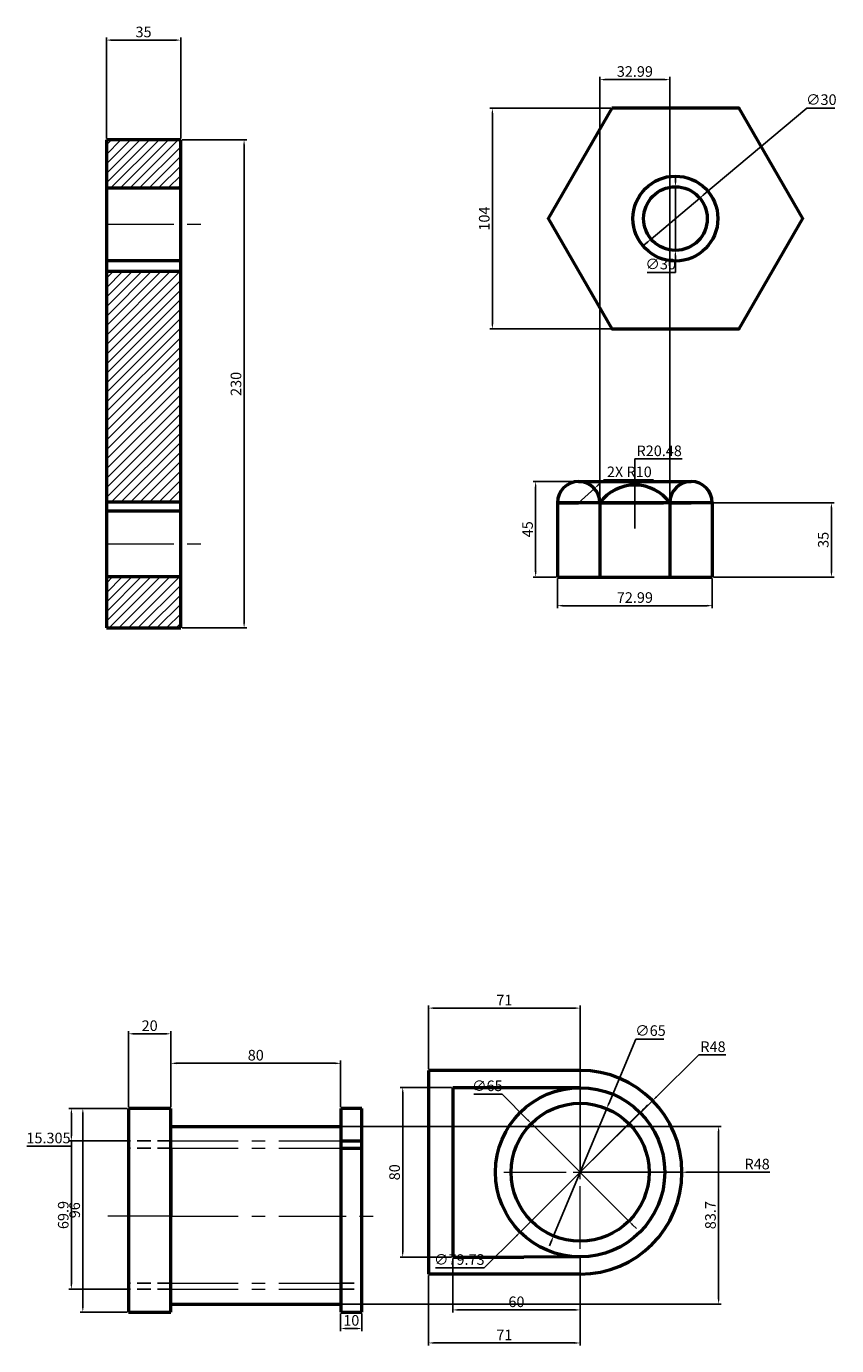
# Model space of a CAD drawing. Units: millimetres. Extents: x 1084 to 2343, y 1141 to 1965.
# Tile 4 of 4: x 1961 to 2343, y 1321 to 1942. Entities that reach past the tile are written whole.
import ezdxf

# ---------------------------------------------------------------- set-up
doc = ezdxf.new("R2010")
doc.units = ezdxf.units.MM
doc.linetypes.add('CENTER', pattern=[50.8, 31.75, -6.35, 6.35, -6.35])
doc.linetypes.add('HIDDEN', pattern=[9.525, 6.35, -3.175])
for name, color, linetype, lineweight in [('M-CNTR', 1, 'CENTER', 18), ('M-DIMS', 2, 'Continuous', 25), ('M-HATC', 8, 'Continuous', 18), ('M-HIDN', 8, 'HIDDEN', 25), ('M-OUTL', 7, 'Continuous', 50)]:
    doc.layers.add(name, color=color, linetype=linetype, lineweight=lineweight)
doc.styles.get("Standard").update_dxf_attribs({"font": 'arial.ttf'})
doc.dimstyles.new('ISO-25', dxfattribs={"dimtxt": 5, "dimasz": 2.5, "dimexe": 1.25, "dimexo": 0.625, "dimtad": 1, "dimtoh": 1, "dimdec": 0, "dimtxsty": 'Standard', "dimcen": 2.5, "dimadec": 0, "dimazin": 0, "dimtfac": 1, "dimtdec": 0, "dimtmove": 0, "dimatfit": 3, "dimfxl": 1, "dimarcsym": 0})

# ---------------------------------------------------------------- blocks, each defined once
blk = doc.blocks.new('*D21')
at = {"layer": 'Defpoints', "color": 0, "transparency": 16777216}
for p in [(2033.5, 1935.59), (1998.5, 1888.61), (2033.5, 1888.61)]:
    blk.add_point(p, dxfattribs=at)
at = {"layer": 'M-DIMS', "color": 0, "lineweight": -2, "transparency": 16777216}
for p, q in [((1998.5, 1889.24), (1998.5, 1936.84)), ((2001, 1935.59), (2031, 1935.59)), ((2033.5, 1889.24), (2033.5, 1936.84))]:
    blk.add_line(p, q, dxfattribs=at)
at = {"layer": 'M-DIMS', "color": 0, "transparency": 16777216}
for points in [[(2001, 1936), (2001, 1935.17), (1998.5, 1935.59)], [(2031, 1936), (2031, 1935.17), (2033.5, 1935.59)]]:
    blk.add_solid(points, dxfattribs=at)
at = {"layer": 'M-DIMS', "color": 0, "transparency": 16777216, "insert": (2016, 1938.77), "char_height": 5, "attachment_point": 5}
blk.add_mtext('35', dxfattribs=at)
blk = doc.blocks.new('*D22')
at = {"layer": 'Defpoints', "color": 0, "transparency": 16777216}
for p in [(2236.62, 1903.46), (2180.37, 1799.54), (2236.62, 1799.54)]:
    blk.add_point(p, dxfattribs=at)
at = {"layer": 'M-DIMS', "color": 0, "lineweight": -2, "transparency": 16777216}
for p, q in [((2236, 1903.46), (2179.12, 1903.46)), ((2180.37, 1900.96), (2180.37, 1802.04)), ((2236, 1799.54), (2179.12, 1799.54))]:
    blk.add_line(p, q, dxfattribs=at)
at = {"layer": 'M-DIMS', "color": 0, "transparency": 16777216}
for points in [[(2179.95, 1900.96), (2180.79, 1900.96), (2180.37, 1903.46)], [(2179.95, 1802.04), (2180.79, 1802.04), (2180.37, 1799.54)]]:
    blk.add_solid(points, dxfattribs=at)
at = {"layer": 'M-DIMS', "color": 0, "transparency": 16777216, "insert": (2177.19, 1851.5), "char_height": 5, "attachment_point": 5, "rotation": 90}
blk.add_mtext('104', dxfattribs=at)
blk = doc.blocks.new('*D23')
at = {"layer": 'Defpoints', "color": 0, "transparency": 16777216}
for p in [(2278.1, 1861.16), (2255.15, 1841.84)]:
    blk.add_point(p, dxfattribs=at)
at = {"layer": 'M-DIMS', "color": 0, "lineweight": -2, "transparency": 16777216}
for p, q in [((2328.46, 1903.58), (2280.01, 1862.77)), ((2341.67, 1903.58), (2328.46, 1903.58)), ((2255.15, 1841.84), (2278.1, 1861.16)), ((2253.24, 1840.23), (2251.33, 1838.62))]:
    blk.add_line(p, q, dxfattribs=at)
at = {"layer": 'M-DIMS', "color": 0, "transparency": 16777216}
for points in [[(2279.74, 1863.09), (2280.28, 1862.46), (2278.1, 1861.16)], [(2252.97, 1840.55), (2253.51, 1839.91), (2255.15, 1841.84)]]:
    blk.add_solid(points, dxfattribs=at)
at = {"layer": 'M-DIMS', "color": 0, "transparency": 16777216, "insert": (2335.37, 1906.89), "char_height": 5, "attachment_point": 5}
blk.add_mtext('∅30', dxfattribs=at)
blk = doc.blocks.new('*D24')
at = {"layer": 'Defpoints', "color": 0, "transparency": 16777216}
for p in [(2221.01, 1727.62), (2200.76, 1682.62), (2211.01, 1682.62)]:
    blk.add_point(p, dxfattribs=at)
at = {"layer": 'M-DIMS', "color": 0, "lineweight": -2, "transparency": 16777216}
for p, q in [((2220.39, 1727.62), (2199.51, 1727.62)), ((2200.76, 1725.12), (2200.76, 1685.12)), ((2210.39, 1682.62), (2199.51, 1682.62))]:
    blk.add_line(p, q, dxfattribs=at)
at = {"layer": 'M-DIMS', "color": 0, "transparency": 16777216}
for points in [[(2200.35, 1725.12), (2201.18, 1725.12), (2200.76, 1727.62)], [(2200.35, 1685.12), (2201.18, 1685.12), (2200.76, 1682.62)]]:
    blk.add_solid(points, dxfattribs=at)
at = {"layer": 'M-DIMS', "color": 0, "transparency": 16777216, "insert": (2197.59, 1705.12), "char_height": 5, "attachment_point": 5, "rotation": 90}
blk.add_mtext('45', dxfattribs=at)
blk = doc.blocks.new('*D38')
at = {"layer": 'Defpoints', "color": 0, "transparency": 16777216}
for p in [(2008.88, 1432.29), (1987.38, 1336.29), (2008.88, 1336.29)]:
    blk.add_point(p, dxfattribs=at)
at = {"layer": 'M-DIMS', "color": 0, "lineweight": -2, "transparency": 16777216}
for p, q in [((2008.26, 1432.29), (1986.13, 1432.29)), ((1987.38, 1429.79), (1987.38, 1338.79)), ((2008.26, 1336.29), (1986.13, 1336.29))]:
    blk.add_line(p, q, dxfattribs=at)
at = {"layer": 'M-DIMS', "color": 0, "transparency": 16777216}
for points in [[(1986.97, 1429.79), (1987.8, 1429.79), (1987.38, 1432.29)], [(1986.97, 1338.79), (1987.8, 1338.79), (1987.38, 1336.29)]]:
    blk.add_solid(points, dxfattribs=at)
at = {"layer": 'M-DIMS', "color": 0, "transparency": 16777216, "insert": (1984.2, 1384.29), "char_height": 5, "attachment_point": 5, "rotation": 90}
blk.add_mtext('96', dxfattribs=at)
blk = doc.blocks.new('*D39')
at = {"layer": 'Defpoints', "color": 0, "transparency": 16777216}
for p in [(2108.88, 1453.51), (2028.88, 1432.29), (2108.88, 1432.29)]:
    blk.add_point(p, dxfattribs=at)
at = {"layer": 'M-DIMS', "color": 0, "lineweight": -2, "transparency": 16777216}
for p, q in [((2028.88, 1432.92), (2028.88, 1454.76)), ((2108.88, 1432.92), (2108.88, 1454.76)), ((2031.38, 1453.51), (2106.38, 1453.51))]:
    blk.add_line(p, q, dxfattribs=at)
at = {"layer": 'M-DIMS', "color": 0, "transparency": 16777216}
for points in [[(2031.38, 1453.93), (2031.38, 1453.09), (2028.88, 1453.51)], [(2106.38, 1453.93), (2106.38, 1453.09), (2108.88, 1453.51)]]:
    blk.add_solid(points, dxfattribs=at)
at = {"layer": 'M-DIMS', "color": 0, "transparency": 16777216, "insert": (2068.88, 1456.69), "char_height": 5, "attachment_point": 5}
blk.add_mtext('80', dxfattribs=at)
blk = doc.blocks.new('*D40')
at = {"layer": 'Defpoints', "color": 0, "transparency": 16777216}
for p in [(2108.88, 1336.29), (2118.88, 1336.29), (2118.88, 1328.57)]:
    blk.add_point(p, dxfattribs=at)
at = {"layer": 'M-DIMS', "color": 0, "lineweight": -2, "transparency": 16777216}
for p, q in [((2108.88, 1335.67), (2108.88, 1327.32)), ((2118.88, 1335.67), (2118.88, 1327.32)), ((2111.38, 1328.57), (2116.38, 1328.57))]:
    blk.add_line(p, q, dxfattribs=at)
at = {"layer": 'M-DIMS', "color": 0, "transparency": 16777216}
for points in [[(2111.38, 1328.98), (2111.38, 1328.15), (2108.88, 1328.57)], [(2116.38, 1328.98), (2116.38, 1328.15), (2118.88, 1328.57)]]:
    blk.add_solid(points, dxfattribs=at)
at = {"layer": 'M-DIMS', "color": 0, "transparency": 16777216, "insert": (2113.88, 1331.75), "char_height": 5, "attachment_point": 5}
blk.add_mtext('10', dxfattribs=at)
blk = doc.blocks.new('*U41')
at = {"layer": 'M-CNTR', "color": 0, "transparency": 16777216}
for p, q in [((0, 6.5), (0, 36)), ((-36, 0), (-6.5, 0)), ((6.5, 0), (36, 0)), ((0, -36), (0, -6.5))]:
    blk.add_line(p, q, dxfattribs=at)
at = {"layer": 'M-CNTR', "color": 0, "linetype": 'Continuous', "transparency": 16777216}
for p, q in [((-3.25, 0), (3.25, 0)), ((0, -3.25), (0, 3.25))]:
    blk.add_line(p, q, dxfattribs=at)
blk = doc.blocks.new('*D42')
at = {"layer": 'Defpoints', "color": 0, "transparency": 16777216}
for p in [(2161.71, 1442.17), (2138.12, 1362.17), (2161.71, 1362.17)]:
    blk.add_point(p, dxfattribs=at)
at = {"layer": 'M-DIMS', "color": 0, "lineweight": -2, "transparency": 16777216}
for p, q in [((2161.08, 1442.17), (2136.87, 1442.17)), ((2138.12, 1439.67), (2138.12, 1364.67)), ((2161.08, 1362.17), (2136.87, 1362.17))]:
    blk.add_line(p, q, dxfattribs=at)
at = {"layer": 'M-DIMS', "color": 0, "transparency": 16777216}
for points in [[(2137.7, 1439.67), (2138.53, 1439.67), (2138.12, 1442.17)], [(2137.7, 1364.67), (2138.53, 1364.67), (2138.12, 1362.17)]]:
    blk.add_solid(points, dxfattribs=at)
at = {"layer": 'M-DIMS', "color": 0, "transparency": 16777216, "insert": (2134.94, 1402.17), "char_height": 5, "attachment_point": 5, "rotation": 90}
blk.add_mtext('80', dxfattribs=at)
blk = doc.blocks.new('*D43')
at = {"layer": 'Defpoints', "color": 0, "transparency": 16777216}
for p in [(2221.71, 1479.52), (2150.32, 1450.17), (2221.71, 1402.17)]:
    blk.add_point(p, dxfattribs=at)
at = {"layer": 'M-DIMS', "color": 0, "lineweight": -2, "transparency": 16777216}
for p, q in [((2150.32, 1450.79), (2150.32, 1480.77)), ((2152.82, 1479.52), (2219.21, 1479.52)), ((2221.71, 1402.79), (2221.71, 1480.77))]:
    blk.add_line(p, q, dxfattribs=at)
at = {"layer": 'M-DIMS', "color": 0, "transparency": 16777216}
for points in [[(2152.82, 1479.93), (2152.82, 1479.1), (2150.32, 1479.52)], [(2219.21, 1479.93), (2219.21, 1479.1), (2221.71, 1479.52)]]:
    blk.add_solid(points, dxfattribs=at)
at = {"layer": 'M-DIMS', "color": 0, "transparency": 16777216, "insert": (2186.01, 1482.65), "char_height": 5, "attachment_point": 5}
blk.add_mtext('71', dxfattribs=at)
blk = doc.blocks.new('*D44')
at = {"layer": 'Defpoints', "color": 0, "transparency": 16777216}
for p in [(2150.32, 1354.17), (2221.71, 1354.17), (2221.71, 1321.76)]:
    blk.add_point(p, dxfattribs=at)
at = {"layer": 'M-DIMS', "color": 0, "lineweight": -2, "transparency": 16777216}
for p, q in [((2150.32, 1353.54), (2150.32, 1320.51)), ((2221.71, 1353.54), (2221.71, 1320.51)), ((2152.82, 1321.76), (2219.21, 1321.76))]:
    blk.add_line(p, q, dxfattribs=at)
at = {"layer": 'M-DIMS', "color": 0, "transparency": 16777216}
for points in [[(2152.82, 1322.17), (2152.82, 1321.34), (2150.32, 1321.76)], [(2219.21, 1322.17), (2219.21, 1321.34), (2221.71, 1321.76)]]:
    blk.add_solid(points, dxfattribs=at)
at = {"layer": 'M-DIMS', "color": 0, "transparency": 16777216, "insert": (2186.01, 1324.89), "char_height": 5, "attachment_point": 5}
blk.add_mtext('71', dxfattribs=at)
blk = doc.blocks.new('*D45')
at = {"layer": 'Defpoints', "color": 0, "transparency": 16777216}
for p in [(2161.71, 1362.17), (2221.71, 1362.3), (2221.71, 1337.33)]:
    blk.add_point(p, dxfattribs=at)
at = {"layer": 'M-DIMS', "color": 0, "lineweight": -2, "transparency": 16777216}
for p, q in [((2161.71, 1361.54), (2161.71, 1336.08)), ((2221.71, 1361.68), (2221.71, 1336.08)), ((2164.21, 1337.33), (2219.21, 1337.33))]:
    blk.add_line(p, q, dxfattribs=at)
at = {"layer": 'M-DIMS', "color": 0, "transparency": 16777216}
for points in [[(2164.21, 1337.75), (2164.21, 1336.91), (2161.71, 1337.33)], [(2219.21, 1337.75), (2219.21, 1336.91), (2221.71, 1337.33)]]:
    blk.add_solid(points, dxfattribs=at)
at = {"layer": 'M-DIMS', "color": 0, "transparency": 16777216, "insert": (2191.71, 1340.51), "char_height": 5, "attachment_point": 5}
blk.add_mtext('60', dxfattribs=at)
blk = doc.blocks.new('*D46')
at = {"layer": 'Defpoints', "color": 0, "transparency": 16777216}
for p in [(2255.85, 1435.9), (2221.71, 1402.17)]:
    blk.add_point(p, dxfattribs=at)
at = {"layer": 'M-DIMS', "color": 0, "lineweight": -2, "transparency": 16777216}
for p, q in [((2277.72, 1457.51), (2257.63, 1437.66)), ((2290.3, 1457.51), (2277.72, 1457.51)), ((2221.71, 1402.17), (2255.85, 1435.9))]:
    blk.add_line(p, q, dxfattribs=at)
at = {"layer": 'M-DIMS', "color": 0, "transparency": 16777216}
blk.add_solid([(2257.34, 1437.96), (2257.92, 1437.37), (2255.85, 1435.9)], dxfattribs=at)
at = {"layer": 'M-DIMS', "color": 0, "transparency": 16777216, "insert": (2284.32, 1460.69), "char_height": 5, "attachment_point": 5}
blk.add_mtext('R48', dxfattribs=at)
blk = doc.blocks.new('*D47')
at = {"layer": 'Defpoints', "color": 0, "transparency": 16777216}
for p in [(2234.22, 1432.16), (2209.2, 1372.17)]:
    blk.add_point(p, dxfattribs=at)
at = {"layer": 'M-DIMS', "color": 0, "lineweight": -2, "transparency": 16777216}
for p, q in [((2247.9, 1464.96), (2235.18, 1434.47)), ((2261.17, 1464.96), (2247.9, 1464.96)), ((2209.2, 1372.17), (2234.22, 1432.16)), ((2208.24, 1369.86), (2207.27, 1367.56))]:
    blk.add_line(p, q, dxfattribs=at)
at = {"layer": 'M-DIMS', "color": 0, "transparency": 16777216}
for points in [[(2234.8, 1434.63), (2235.57, 1434.31), (2234.22, 1432.16)], [(2207.85, 1370.02), (2208.62, 1369.7), (2209.2, 1372.17)]]:
    blk.add_solid(points, dxfattribs=at)
at = {"layer": 'M-DIMS', "color": 0, "transparency": 16777216, "insert": (2254.85, 1468.28), "char_height": 5, "attachment_point": 5}
blk.add_mtext('∅65', dxfattribs=at)
blk = doc.blocks.new('*D58')
at = {"layer": 'Defpoints', "color": 0, "transparency": 16777216}
for p in [(2033.5, 1888.61), (2033.5, 1658.61), (2063.38, 1658.61)]:
    blk.add_point(p, dxfattribs=at)
at = {"layer": 'M-DIMS', "color": 0, "lineweight": -2, "transparency": 16777216}
for p, q in [((2034.13, 1888.61), (2064.63, 1888.61)), ((2063.38, 1886.11), (2063.38, 1661.11)), ((2034.13, 1658.61), (2064.63, 1658.61))]:
    blk.add_line(p, q, dxfattribs=at)
at = {"layer": 'M-DIMS', "color": 0, "transparency": 16777216}
for points in [[(2062.96, 1886.11), (2063.79, 1886.11), (2063.38, 1888.61)], [(2062.96, 1661.11), (2063.79, 1661.11), (2063.38, 1658.61)]]:
    blk.add_solid(points, dxfattribs=at)
at = {"layer": 'M-DIMS', "color": 0, "transparency": 16777216, "insert": (2060.2, 1773.61), "char_height": 5, "attachment_point": 5, "rotation": 90}
blk.add_mtext('230', dxfattribs=at)
blk = doc.blocks.new('*D59')
at = {"layer": 'Defpoints', "color": 0, "transparency": 16777216}
for p in [(2211.01, 1682.62), (2284, 1682.62), (2284, 1669.12)]:
    blk.add_point(p, dxfattribs=at)
at = {"layer": 'M-DIMS', "color": 0, "lineweight": -2, "transparency": 16777216}
for p, q in [((2211.01, 1682), (2211.01, 1667.87)), ((2284, 1682), (2284, 1667.87)), ((2213.51, 1669.12), (2281.5, 1669.12))]:
    blk.add_line(p, q, dxfattribs=at)
at = {"layer": 'M-DIMS', "color": 0, "transparency": 16777216}
for points in [[(2213.51, 1669.54), (2213.51, 1668.71), (2211.01, 1669.12)], [(2281.5, 1669.54), (2281.5, 1668.71), (2284, 1669.12)]]:
    blk.add_solid(points, dxfattribs=at)
at = {"layer": 'M-DIMS', "color": 0, "transparency": 16777216, "insert": (2247.51, 1672.3), "char_height": 5, "attachment_point": 5}
blk.add_mtext('72.99', dxfattribs=at)
blk = doc.blocks.new('*D60')
at = {"layer": 'Defpoints', "color": 0, "transparency": 16777216}
for p in [(2264, 1916.96), (2231.01, 1717.62), (2264, 1717.62)]:
    blk.add_point(p, dxfattribs=at)
at = {"layer": 'M-DIMS', "color": 0, "lineweight": -2, "transparency": 16777216}
for p, q in [((2231.01, 1718.25), (2231.01, 1918.21)), ((2233.51, 1916.96), (2261.5, 1916.96)), ((2264, 1718.25), (2264, 1918.21))]:
    blk.add_line(p, q, dxfattribs=at)
at = {"layer": 'M-DIMS', "color": 0, "transparency": 16777216}
for points in [[(2233.51, 1917.38), (2233.51, 1916.55), (2231.01, 1916.96)], [(2261.5, 1917.38), (2261.5, 1916.55), (2264, 1916.96)]]:
    blk.add_solid(points, dxfattribs=at)
at = {"layer": 'M-DIMS', "color": 0, "transparency": 16777216, "insert": (2247.51, 1920.14), "char_height": 5, "attachment_point": 5}
blk.add_mtext('32.99', dxfattribs=at)
blk = doc.blocks.new('*D61')
at = {"layer": 'Defpoints', "color": 0, "transparency": 16777216}
for p in [(2284, 1717.62), (2340.12, 1717.62), (2284, 1682.62)]:
    blk.add_point(p, dxfattribs=at)
at = {"layer": 'M-DIMS', "color": 0, "lineweight": -2, "transparency": 16777216}
for p, q in [((2284.62, 1717.62), (2341.37, 1717.62)), ((2340.12, 1685.12), (2340.12, 1715.12)), ((2284.62, 1682.62), (2341.37, 1682.62))]:
    blk.add_line(p, q, dxfattribs=at)
at = {"layer": 'M-DIMS', "color": 0, "transparency": 16777216}
for points in [[(2339.71, 1715.12), (2340.54, 1715.12), (2340.12, 1717.62)], [(2339.71, 1685.12), (2340.54, 1685.12), (2340.12, 1682.62)]]:
    blk.add_solid(points, dxfattribs=at)
at = {"layer": 'M-DIMS', "color": 0, "transparency": 16777216, "insert": (2336.95, 1700.12), "char_height": 5, "attachment_point": 5, "rotation": 90}
blk.add_mtext('35', dxfattribs=at)
blk = doc.blocks.new('*D65')
at = {"layer": 'Defpoints', "color": 0, "transparency": 16777216}
for p in [(2028.88, 1467.42), (2008.88, 1432.29), (2028.88, 1432.29)]:
    blk.add_point(p, dxfattribs=at)
at = {"layer": 'M-DIMS', "color": 0, "lineweight": -2, "transparency": 16777216}
for p, q in [((2008.88, 1432.92), (2008.88, 1468.67)), ((2011.38, 1467.42), (2026.38, 1467.42)), ((2028.88, 1432.92), (2028.88, 1468.67))]:
    blk.add_line(p, q, dxfattribs=at)
at = {"layer": 'M-DIMS', "color": 0, "transparency": 16777216}
for points in [[(2011.38, 1467.83), (2011.38, 1467), (2008.88, 1467.42)], [(2026.38, 1467.83), (2026.38, 1467), (2028.88, 1467.42)]]:
    blk.add_solid(points, dxfattribs=at)
at = {"layer": 'M-DIMS', "color": 0, "transparency": 16777216, "insert": (2018.88, 1470.59), "char_height": 5, "attachment_point": 5}
blk.add_mtext('20', dxfattribs=at)
blk = doc.blocks.new('*D66')
at = {"layer": 'Defpoints', "color": 0, "transparency": 16777216}
for p in [(2008.88, 1432.29), (1981.99, 1416.99), (2008.88, 1416.99)]:
    blk.add_point(p, dxfattribs=at)
at = {"layer": 'M-DIMS', "color": 0, "lineweight": -2, "transparency": 16777216}
for p, q in [((2008.26, 1432.29), (1980.74, 1432.29)), ((1981.99, 1429.79), (1981.99, 1419.49)), ((1981.99, 1414.49), (1961.04, 1414.49)), ((2008.26, 1416.99), (1980.74, 1416.99)), ((1981.99, 1416.99), (1981.99, 1414.49))]:
    blk.add_line(p, q, dxfattribs=at)
at = {"layer": 'M-DIMS', "color": 0, "transparency": 16777216}
for points in [[(1981.58, 1429.79), (1982.41, 1429.79), (1981.99, 1432.29)], [(1981.58, 1419.49), (1982.41, 1419.49), (1981.99, 1416.99)]]:
    blk.add_solid(points, dxfattribs=at)
at = {"layer": 'M-DIMS', "color": 0, "transparency": 16777216, "insert": (1971.21, 1417.67), "char_height": 5, "attachment_point": 5}
blk.add_mtext('15.305', dxfattribs=at)
blk = doc.blocks.new('*D67')
at = {"layer": 'Defpoints', "color": 0, "transparency": 16777216}
for p in [(2008.88, 1416.99), (1981.99, 1347.08), (2008.88, 1347.08)]:
    blk.add_point(p, dxfattribs=at)
at = {"layer": 'M-DIMS', "color": 0, "lineweight": -2, "transparency": 16777216}
for p, q in [((2008.26, 1416.99), (1980.74, 1416.99)), ((1981.99, 1414.49), (1981.99, 1349.58)), ((2008.26, 1347.08), (1980.74, 1347.08))]:
    blk.add_line(p, q, dxfattribs=at)
at = {"layer": 'M-DIMS', "color": 0, "transparency": 16777216}
for points in [[(1981.58, 1414.49), (1982.41, 1414.49), (1981.99, 1416.99)], [(1981.58, 1349.58), (1982.41, 1349.58), (1981.99, 1347.08)]]:
    blk.add_solid(points, dxfattribs=at)
at = {"layer": 'M-DIMS', "color": 0, "transparency": 16777216, "insert": (1978.81, 1382.03), "char_height": 5, "attachment_point": 5, "rotation": 90}
blk.add_mtext('69.9', dxfattribs=at)
blk = doc.blocks.new('*D68')
at = {"layer": 'Defpoints', "color": 0, "transparency": 16777216}
for p in [(2108.88, 1423.81), (2108.88, 1340.11), (2286.96, 1340.11)]:
    blk.add_point(p, dxfattribs=at)
at = {"layer": 'M-DIMS', "color": 0, "lineweight": -2, "transparency": 16777216}
for p, q in [((2109.51, 1423.81), (2288.21, 1423.81)), ((2286.96, 1421.31), (2286.96, 1342.61)), ((2109.51, 1340.11), (2288.21, 1340.11))]:
    blk.add_line(p, q, dxfattribs=at)
at = {"layer": 'M-DIMS', "color": 0, "transparency": 16777216}
for points in [[(2286.54, 1421.31), (2287.38, 1421.31), (2286.96, 1423.81)], [(2286.54, 1342.61), (2287.38, 1342.61), (2286.96, 1340.11)]]:
    blk.add_solid(points, dxfattribs=at)
at = {"layer": 'M-DIMS', "color": 0, "transparency": 16777216, "insert": (2283.78, 1381.96), "char_height": 5, "attachment_point": 5, "rotation": 90}
blk.add_mtext('83.7', dxfattribs=at)
blk = doc.blocks.new('*D74')
at = {"layer": 'Defpoints', "color": 0, "transparency": 16777216}
for p in [(2266.65, 1866.5), (2266.6, 1836.5)]:
    blk.add_point(p, dxfattribs=at)
at = {"layer": 'M-DIMS', "color": 0, "lineweight": -2, "transparency": 16777216}
for p, q in [((2266.65, 1869), (2266.66, 1871.5)), ((2266.65, 1866.5), (2266.6, 1836.5)), ((2266.58, 1826.12), (2266.6, 1834)), ((2253.37, 1826.12), (2266.58, 1826.12))]:
    blk.add_line(p, q, dxfattribs=at)
at = {"layer": 'M-DIMS', "color": 0, "transparency": 16777216}
for points in [[(2266.24, 1869), (2267.07, 1869), (2266.65, 1866.5)], [(2266.18, 1834), (2267.01, 1834), (2266.6, 1836.5)]]:
    blk.add_solid(points, dxfattribs=at)
at = {"layer": 'M-DIMS', "color": 0, "transparency": 16777216, "insert": (2259.67, 1829.43), "char_height": 5, "attachment_point": 5}
blk.add_mtext('∅30', dxfattribs=at)
blk = doc.blocks.new('*D75')
at = {"layer": 'Defpoints', "color": 0, "transparency": 16777216}
for p in [(2247.51, 1725.96), (2247.51, 1705.48)]:
    blk.add_point(p, dxfattribs=at)
at = {"layer": 'M-DIMS', "color": 0, "lineweight": -2, "transparency": 16777216}
for p, q in [((2269.81, 1738.25), (2247.51, 1738.25)), ((2247.51, 1738.25), (2247.51, 1728.46)), ((2247.51, 1705.48), (2247.51, 1725.96))]:
    blk.add_line(p, q, dxfattribs=at)
at = {"layer": 'M-DIMS', "color": 0, "transparency": 16777216}
blk.add_solid([(2247.09, 1728.46), (2247.93, 1728.46), (2247.51, 1725.96)], dxfattribs=at)
at = {"layer": 'M-DIMS', "color": 0, "transparency": 16777216, "insert": (2258.97, 1741.43), "char_height": 5, "attachment_point": 5}
blk.add_mtext('R20.48', dxfattribs=at)
blk = doc.blocks.new('*D76')
at = {"layer": 'Defpoints', "color": 0, "transparency": 16777216}
for p in [(2228.44, 1724.32), (2221.01, 1717.62)]:
    blk.add_point(p, dxfattribs=at)
at = {"layer": 'M-DIMS', "color": 0, "lineweight": -2, "transparency": 16777216}
for p, q in [((2232.89, 1728.34), (2230.29, 1726)), ((2256.28, 1728.34), (2232.89, 1728.34)), ((2221.01, 1717.62), (2228.44, 1724.32))]:
    blk.add_line(p, q, dxfattribs=at)
at = {"layer": 'M-DIMS', "color": 0, "transparency": 16777216}
blk.add_solid([(2230.01, 1726.31), (2230.57, 1725.69), (2228.44, 1724.32)], dxfattribs=at)
at = {"layer": 'M-DIMS', "color": 0, "transparency": 16777216, "insert": (2244.9, 1731.52), "char_height": 5, "attachment_point": 5}
blk.add_mtext('2X R10', dxfattribs=at)
blk = doc.blocks.new('*D78')
at = {"layer": 'Defpoints', "color": 0, "transparency": 16777216}
for p in [(2198.74, 1425.16), (2244.68, 1379.17)]:
    blk.add_point(p, dxfattribs=at)
at = {"layer": 'M-DIMS', "color": 0, "lineweight": -2, "transparency": 16777216}
for p, q in [((2171.69, 1438.96), (2184.96, 1438.96)), ((2184.96, 1438.96), (2196.97, 1426.93)), ((2244.68, 1379.17), (2198.74, 1425.16)), ((2246.44, 1377.41), (2248.21, 1375.64))]:
    blk.add_line(p, q, dxfattribs=at)
at = {"layer": 'M-DIMS', "color": 0, "transparency": 16777216}
for points in [[(2197.27, 1427.22), (2196.68, 1426.63), (2198.74, 1425.16)], [(2246.74, 1377.7), (2246.15, 1377.11), (2244.68, 1379.17)]]:
    blk.add_solid(points, dxfattribs=at)
at = {"layer": 'M-DIMS', "color": 0, "transparency": 16777216, "insert": (2178.01, 1442.27), "char_height": 5, "attachment_point": 5}
blk.add_mtext('∅65', dxfattribs=at)
blk = doc.blocks.new('*D79')
at = {"layer": 'Defpoints', "color": 0, "transparency": 16777216}
for p in [(2249.92, 1430.33), (2193.5, 1374)]:
    blk.add_point(p, dxfattribs=at)
at = {"layer": 'M-DIMS', "color": 0, "lineweight": -2, "transparency": 16777216}
for p, q in [((2249.92, 1430.33), (2193.5, 1374)), ((2251.69, 1432.1), (2253.46, 1433.87)), ((2176.57, 1357.1), (2191.73, 1372.23)), ((2153.64, 1357.1), (2176.57, 1357.1))]:
    blk.add_line(p, q, dxfattribs=at)
at = {"layer": 'M-DIMS', "color": 0, "transparency": 16777216}
for points in [[(2251.39, 1432.4), (2251.98, 1431.81), (2249.92, 1430.33)], [(2191.44, 1372.53), (2192.02, 1371.94), (2193.5, 1374)]]:
    blk.add_solid(points, dxfattribs=at)
at = {"layer": 'M-DIMS', "color": 0, "transparency": 16777216, "insert": (2164.79, 1360.42), "char_height": 5, "attachment_point": 5}
blk.add_mtext('∅79.73', dxfattribs=at)
blk = doc.blocks.new('*D80')
at = {"layer": 'Defpoints', "color": 0, "transparency": 16777216}
for p in [(2221.71, 1402.17), (2269.71, 1402.2)]:
    blk.add_point(p, dxfattribs=at)
at = {"layer": 'M-DIMS', "color": 0, "lineweight": -2, "transparency": 16777216}
for p, q in [((2221.71, 1402.17), (2269.71, 1402.2)), ((2298.51, 1402.22), (2272.21, 1402.2)), ((2311.09, 1402.22), (2298.51, 1402.22))]:
    blk.add_line(p, q, dxfattribs=at)
at = {"layer": 'M-DIMS', "color": 0, "transparency": 16777216}
blk.add_solid([(2272.21, 1402.62), (2272.21, 1401.79), (2269.71, 1402.2)], dxfattribs=at)
at = {"layer": 'M-DIMS', "color": 0, "transparency": 16777216, "insert": (2305.11, 1405.4), "char_height": 5, "attachment_point": 5}
blk.add_mtext('R48', dxfattribs=at)

msp = doc.modelspace()

# ---------------------------------------------------------------- hatches: boundary and pattern name
at = {"layer": 'M-HATC'}
h = msp.add_hatch(dxfattribs=at)
h.set_pattern_fill('ANSI31', color=256)
h.paths.add_polyline_path([(2033.504, 1888.614), (1998.504, 1888.614), (1998.504, 1865.7878), (2033.504, 1865.7878)])
h.paths.add_polyline_path([(2033.504, 1826.5296), (1998.504, 1826.5296), (1998.504, 1718.092), (2033.504, 1718.092)])
h.paths.add_polyline_path([(2033.504, 1682.7931), (1998.504, 1682.7931), (1998.504, 1658.614), (2033.504, 1658.614)])

# ---------------------------------------------------------------- linework, layer by layer
at = {"layer": 'M-CNTR'}
for p, q in [((1998.504, 1865.7878), (1998.504, 1848.7878)), ((1998.504, 1848.7878), (2047.3771, 1848.7878)), ((1998.504, 1713.7349), (1998.504, 1698.2349)), ((1998.504, 1698.2349), (2043.1832, 1698.2349)), ((2028.8828, 1416.986), (2108.8828, 1416.986)), ((2028.8828, 1413.5171), (2108.8828, 1413.5171)), ((2028.8828, 1381.5171), (1999.2425, 1381.5171)), ((2028.8828, 1381.5171), (2124.9789, 1381.5171)), ((2028.8828, 1349.9794), (2108.8828, 1349.9794)), ((2028.8828, 1347.0819), (2108.8828, 1347.0819))]:
    msp.add_line(p, q, dxfattribs=at)
at = {"layer": 'M-HIDN'}
for p, q in [((2028.8828, 1416.986), (2008.8828, 1416.986)), ((2028.8828, 1413.5171), (2008.8828, 1413.5171)), ((2028.8828, 1349.9794), (2008.8828, 1349.9794)), ((2108.8828, 1349.9794), (2118.8828, 1349.9794)), ((2028.8828, 1347.0819), (2008.8828, 1347.0819)), ((2108.8828, 1347.0819), (2118.8828, 1347.0819))]:
    msp.add_line(p, q, dxfattribs=at)
at = {"layer": 'M-OUTL'}
for p, q in [((1998.504, 1888.614), (1998.504, 1658.614)), ((2033.504, 1888.614), (1998.504, 1888.614)), ((2033.504, 1658.614), (2033.504, 1888.614)), ((2033.504, 1865.7878), (1998.504, 1865.7878)), ((2033.504, 1831.5995), (1998.504, 1831.5995)), ((2033.504, 1826.5296), (1998.504, 1826.5296)), ((2221.0123, 1727.6241), (2273.9996, 1727.6241)), ((1998.504, 1718.092), (2033.504, 1718.092)), ((2211.0123, 1717.6241), (2211.0123, 1682.6241)), ((2283.9996, 1717.6241), (2211.0123, 1717.6241)), ((2211.0123, 1717.6241), (2221.0123, 1717.6241)), ((2231.0123, 1717.6241), (2261.0123, 1717.6241)), ((2231.0123, 1717.6241), (2231.0123, 1682.6241)), ((2263.9996, 1717.6241), (2273.9996, 1717.6241)), ((2263.9996, 1717.6241), (2263.9996, 1682.6241)), ((2283.9996, 1717.6241), (2283.9996, 1682.6241)), ((1998.504, 1713.7349), (2033.504, 1713.7349)), ((1998.504, 1682.7931), (2033.504, 1682.7931)), ((2211.0123, 1682.6241), (2283.9996, 1682.6241)), ((1998.504, 1658.614), (2033.504, 1658.614)), ((2221.709, 1450.1669), (2150.3163, 1450.1669)), ((2150.3163, 1450.1669), (2150.3163, 1354.1669)), ((2161.709, 1442.1669), (2161.709, 1362.1669)), ((2161.709, 1442.1669), (2221.709, 1442.1669)), ((2221.709, 1442.1669), (2221.709, 1442.0311)), ((2008.8828, 1432.2906), (2008.8828, 1336.2906)), ((2028.8828, 1432.2906), (2008.8828, 1432.2906)), ((2028.8828, 1336.2906), (2028.8828, 1432.2906)), ((2108.8828, 1432.2906), (2108.8828, 1336.2906)), ((2118.8828, 1432.2906), (2108.8828, 1432.2906)), ((2118.8828, 1336.2906), (2118.8828, 1432.2906)), ((2028.8828, 1423.812), (2108.8828, 1423.812)), ((2028.8828, 1413.5171), (2028.8828, 1381.5171)), ((2108.8828, 1416.986), (2118.8828, 1416.986)), ((2108.8828, 1413.5171), (2118.8828, 1413.5171)), ((2161.709, 1362.1669), (2195.176, 1362.1669)), ((2221.709, 1362.3026), (2195.176, 1362.1669)), ((2221.709, 1354.1669), (2150.3163, 1354.1669)), ((2028.8828, 1340.1061), (2108.8828, 1340.1061)), ((2008.8828, 1336.2906), (2028.8828, 1336.2906)), ((2108.8828, 1336.2906), (2118.8828, 1336.2906))]:
    msp.add_line(p, q, dxfattribs=at)
msp.add_lwpolyline([(2236.6249, 1903.4619), (2206.6249, 1851.5004), (2236.6249, 1799.5389), (2296.6249, 1799.5389), (2326.6249, 1851.5004), (2296.6249, 1903.4619)], close=True, dxfattribs=at)
for centre, radius in [((2266.6249, 1851.5004), 20), ((2266.6249, 1851.5004), 15), ((2221.709, 1402.1669), 39.8643), ((2221.709, 1402.1669), 32.5)]:
    msp.add_circle(centre, radius, dxfattribs=at)
for centre, radius, start, end in [((2221.0123, 1717.6241), 10, 0, 180), ((2247.506, 1705.4843), 20.4796, 36.3540258, 143.6459742), ((2273.9996, 1717.6241), 10, 0, 180), ((2221.709, 1402.1669), 48, 270, 90)]:
    msp.add_arc(centre, radius, start, end, dxfattribs=at)

# ---------------------------------------------------------------- block references
at = {"layer": 'M-CNTR'}
msp.add_blockref('*U41', (2221.709, 1402.1669), dxfattribs=at)

# ---------------------------------------------------------------- dimensions: what is measured, and where the dimension line sits
at = {"layer": 'M-DIMS'}
for base, p1, p2, override, picture, middle in [((2033.504, 1935.5879), (1998.504, 1888.614), (2033.504, 1888.614), {"dimclrd": 0, "dimclre": 0, "dimclrt": 0}, '*D21', (2016.004, 1938.7674)), ((2263.9996, 1916.9619), (2231.0123, 1717.6241), (2263.9996, 1717.6241), {"dimdec": 2, "dimlfac": 1, "dimrnd": 0, "dimzin": 0, "dimdsep": 46, "dimlunit": 2}, '*D60', (2247.506, 1920.1415)), ((2283.9996, 1669.1241), (2211.0123, 1682.6241), (2283.9996, 1682.6241), {"dimdec": 2, "dimlfac": 1, "dimrnd": 0, "dimzin": 0, "dimdsep": 46, "dimlunit": 2}, '*D59', (2247.506, 1672.3019)), ((2221.709, 1479.516), (2150.3163, 1450.1669), (2221.709, 1402.1669), {"dimclrd": 0, "dimclre": 0, "dimclrt": 0}, '*D43', (2186.0126, 1482.6512)), ((2028.8828, 1467.4169), (2008.8828, 1432.2906), (2028.8828, 1432.2906), {"dimdec": 0, "dimlfac": 1, "dimrnd": 0, "dimzin": 0, "dimdsep": 46, "dimlunit": 2}, '*D65', (2018.8828, 1470.5947)), ((2108.8828, 1453.5097), (2028.8828, 1432.2906), (2108.8828, 1432.2906), {"dimclrd": 0, "dimclre": 0, "dimclrt": 0}, '*D39', (2068.8828, 1456.6875)), ((2221.709, 1337.3286), (2161.709, 1362.1669), (2221.709, 1362.3026), {"dimclrd": 0, "dimclre": 0, "dimclrt": 0}, '*D45', (2191.709, 1340.5064)), ((2221.709, 1321.7557), (2150.3163, 1354.1669), (2221.709, 1354.1669), {"dimclrd": 0, "dimclre": 0, "dimclrt": 0}, '*D44', (2186.0126, 1324.8909)), ((2118.8828, 1328.5673), (2108.8828, 1336.2906), (2118.8828, 1336.2906), {"dimclrd": 0, "dimclre": 0, "dimclrt": 0}, '*D40', (2113.8828, 1331.7452))]:
    dim = msp.add_linear_dim(base=base, p1=p1, p2=p2, dimstyle='ISO-25', override=override, dxfattribs=at)
    dim.commit()
    dim.dimension.update_dxf_attribs({"geometry": picture, "text_midpoint": middle})
for p1, p2, override, picture, middle in [((2255.1519, 1841.8376), (2278.0979, 1861.1632), {"dimclrd": 0, "dimclre": 0, "dimclrt": 0}, '*D23', (2335.3748, 1903.577)), ((2266.6497, 1866.5004), (2266.6002, 1836.5004), {"dimdec": 0, "dimlfac": 1, "dimrnd": 0, "dimzin": 0, "dimdsep": 46, "dimlunit": 2}, '*D74', (2259.6654, 1826.115)), ((2209.1975, 1372.1717), (2234.2205, 1432.1621), {"dimclrd": 0, "dimclre": 0, "dimclrt": 0}, '*D47', (2254.8453, 1464.9587)), ((2244.6779, 1379.1739), (2198.7401, 1425.1599), {"dimdec": 0, "dimlfac": 1, "dimrnd": 0, "dimzin": 0, "dimdsep": 46, "dimlunit": 2}, '*D78', (2178.0138, 1438.9557)), ((2249.9183, 1430.3341), (2193.4997, 1373.9997), {"dimdec": 2, "dimlfac": 1, "dimrnd": 0, "dimzin": 0, "dimdsep": 46, "dimlunit": 2}, '*D79', (2164.7929, 1357.0993))]:
    dim = msp.add_diameter_dim_2p(p1=p1, p2=p2, dimstyle='ISO-25', override=override, dxfattribs=at)
    dim.commit()
    dim.dimension.update_dxf_attribs({"geometry": picture, "text_midpoint": middle, "dimtype": 163})
for base, p1, p2, override, picture, middle in [((2180.3703, 1799.5389), (2236.6249, 1903.4619), (2236.6249, 1799.5389), {"dimclrd": 0, "dimclre": 0, "dimclrt": 0}, '*D22', (2177.1925, 1851.5004)), ((2063.3771, 1658.614), (2033.504, 1888.614), (2033.504, 1658.614), {"dimdec": 0, "dimlfac": 1, "dimrnd": 0, "dimzin": 0, "dimdsep": 46, "dimlunit": 2}, '*D58', (2060.1975, 1773.614)), ((2200.7622, 1682.6241), (2221.0123, 1727.6241), (2211.0123, 1682.6241), {"dimclrd": 0, "dimclre": 0, "dimclrt": 0}, '*D24', (2197.5946, 1705.1241)), ((2340.1249, 1717.6241), (2283.9996, 1682.6241), (2283.9996, 1717.6241), {"dimdec": 0, "dimlfac": 1, "dimrnd": 0, "dimzin": 0, "dimdsep": 46, "dimlunit": 2}, '*D61', (2336.9453, 1700.1241)), ((2138.1171, 1362.1669), (2161.709, 1442.1669), (2161.709, 1362.1669), {"dimclrd": 0, "dimclre": 0, "dimclrt": 0}, '*D42', (2134.9392, 1402.1669)), ((1981.9925, 1416.986), (2008.8828, 1432.2906), (2008.8828, 1416.986), {"dimdec": 3, "dimlfac": 1, "dimrnd": 0, "dimzin": 0, "dimdsep": 46, "dimlunit": 2}, '*D66', (1971.2055, 1417.6656)), ((1987.3827, 1336.2906), (2008.8828, 1432.2906), (2008.8828, 1336.2906), {"dimclrd": 0, "dimclre": 0, "dimclrt": 0}, '*D38', (1984.2049, 1384.2906)), ((2286.959, 1340.1061), (2108.8828, 1423.812), (2108.8828, 1340.1061), {"dimdec": 1, "dimlfac": 1, "dimrnd": 0, "dimzin": 0, "dimdsep": 46, "dimlunit": 2}, '*D68', (2283.7794, 1381.959)), ((1981.9925, 1347.0819), (2008.8828, 1416.986), (2008.8828, 1347.0819), {"dimdec": 1, "dimlfac": 1, "dimrnd": 0, "dimzin": 0, "dimdsep": 46, "dimlunit": 2}, '*D67', (1978.8146, 1382.034))]:
    dim = msp.add_linear_dim(base=base, p1=p1, p2=p2, angle=90, dimstyle='ISO-25', override=override, dxfattribs=at)
    dim.commit()
    dim.dimension.update_dxf_attribs({"geometry": picture, "text_midpoint": middle})
for center, mpoint, override, picture, middle in [((2247.506, 1705.4843), (2247.51, 1725.9639), {"dimdec": 2, "dimlfac": 1, "dimrnd": 0, "dimzin": 0, "dimdsep": 46, "dimlunit": 2}, '*D75', (2258.9713, 1738.2517)), ((2221.709, 1402.1669), (2255.8523, 1435.9047), {"dimclrd": 0, "dimclre": 0, "dimclrt": 0}, '*D46', (2284.3219, 1457.5108)), ((2221.709, 1402.1669), (2269.709, 1402.2), {"dimdec": 0, "dimlfac": 1, "dimrnd": 0, "dimzin": 0, "dimdsep": 46, "dimlunit": 2}, '*D80', (2298.509, 1402.2199))]:
    dim = msp.add_radius_dim(center=center, mpoint=mpoint, dimstyle='ISO-25', override=override, dxfattribs=at)
    dim.commit()
    dim.dimension.update_dxf_attribs({"geometry": picture, "text_midpoint": middle, "dimtype": 164})
dim = msp.add_radius_dim(center=(2221.0123, 1717.6241), mpoint=(2228.4366, 1724.3233), text='2X <>', dimstyle='ISO-25', override={"dimdec": 0, "dimlfac": 1, "dimrnd": 0, "dimzin": 0, "dimdsep": 46, "dimlunit": 2}, dxfattribs=at)
dim.commit()
dim.dimension.update_dxf_attribs({"geometry": '*D76', "text_midpoint": (2244.8958, 1728.3428), "dimtype": 164})

doc.saveas('drawing.dxf')
